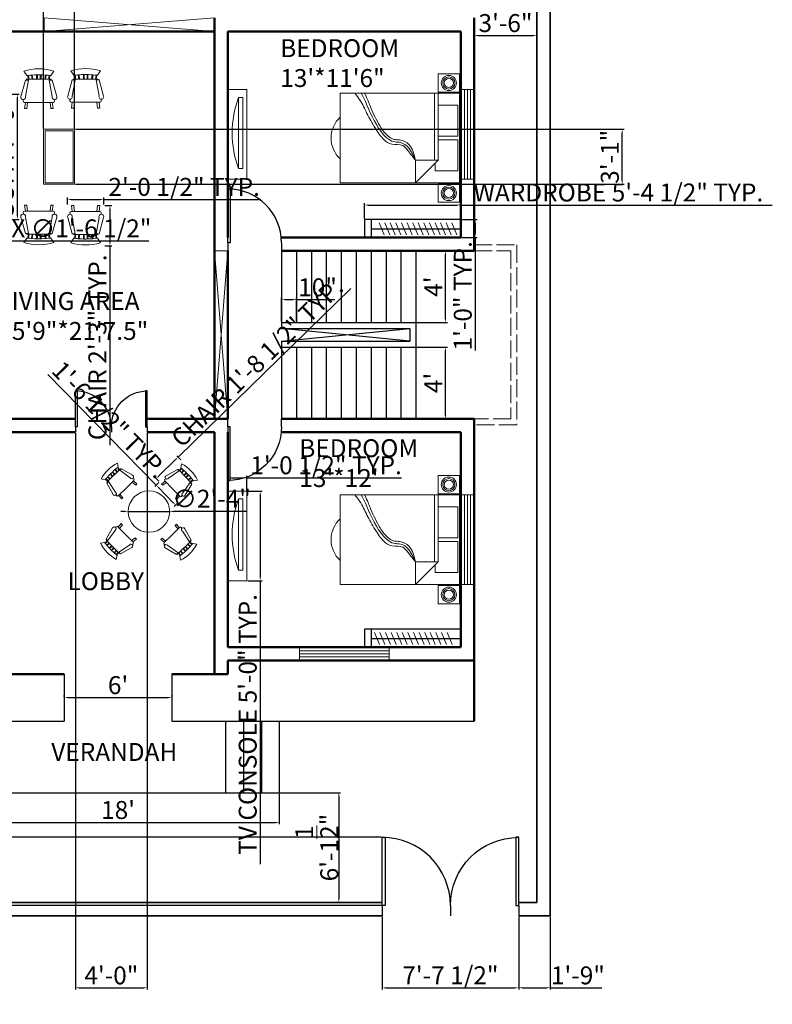
# Model space of a CAD drawing. Units: inches. Extents: x 6286 to 7213, y 5725 to 6776.
# Tile 3 of 5: x 6709 to 7213, y 5725 to 6385. Entities that reach past the tile are written whole.
import ezdxf

# ---------------------------------------------------------------- set-up
doc = ezdxf.new("R2010")
doc.units = ezdxf.units.IN
doc.linetypes.add('ACAD_ISO02W100', pattern=[15, 12, -3])
for name, color, linetype, lineweight in [('A-ANNO-DIMS', 2, 'Continuous', 18), ('A-AREA-IDEN', 7, 'Continuous', 25), ('A-DOOR', 3, 'Continuous', 25), ('A-FLOR', 7, 'Continuous', 25), ('A-FLOR-CASE', 8, 'Continuous', 25), ('A-FLOR-CASE-PATT', 252, 'Continuous', 13), ('A-FLOR-STRS', 7, 'Continuous', 25), ('A-FLOR-STRS-HIDN', 8, 'ACAD_ISO02W100', 18), ('A-FURN', 8, 'Continuous', 18), ('A-GLAZ', 4, 'Continuous', 18), ('A-WALL', 7, 'Continuous', 50), ('A-WALL-OPEN', 7, 'Continuous', 18), ('C-PROP', 7, 'Continuous', 35), ('L-SITE-GATE', 3, 'Continuous', 25)]:
    doc.layers.add(name, color=color, linetype=linetype, lineweight=lineweight)
doc.styles.get("Standard").update_dxf_attribs({"font": 'arial.ttf'})
doc.dimstyles.new('ISO-25', dxfattribs={"dimtxt": 12, "dimasz": 2.5, "dimexe": 1.25, "dimexo": 0.625, "dimtad": 1, "dimdec": 1, "dimlunit": 4, "dimtxsty": 'Standard', "dimcen": 2.5, "dimadec": 0, "dimazin": 0, "dimtfac": 1, "dimtdec": 1, "dimtmove": 0, "dimatfit": 3, "dimfxl": 1, "dimarcsym": 0})

# ---------------------------------------------------------------- blocks, each defined once
blk = doc.blocks.new('Chair - Rocking')
for p, q in [((-8, -4.5), (-10, -1.5)), ((-7.5, -4.5), (-7, -7)), ((-6.5, -7), (-7.02225, -4.43)), ((-4.5, -7), (-4.96674, -4.19951)), ((-4, -7), (-4.40532, -4.16272)), ((-1.5, -4.05012), (-1.5, -7)), ((-1, -7), (-1, -4.05012)), ((1, -7), (1, -4.04655)), ((1.5, -4.05012), (1.5, -7)), ((4, -7), (4.40187, -4.18694)), ((4.5, -7), (4.96761, -4.19437)), ((6.5, -7), (7, -4.4057)), ((7.5, -4.5), (7, -7)), ((8, -4.5), (10, -1.5)), ((-9, -7.5), (-12, -18.49999)), ((-7, -7.5), (-9, -7.5)), ((-9, -18.49999), (-7, -7.5)), ((-8.23428, -6.99939), (-8.3093, -7.47958)), ((-8.23041, -7), (8.23915, -7)), ((7, -7.5), (9, -7.5)), ((9, -18.49999), (7, -7.5)), ((8.31071, -7.48854), (8.23449, -7.00073)), ((9, -7.5), (12, -18.49999)), ((-10.36644, -20.64523), (-10.5, -21.49999)), ((-9, -22.49999), (-9.5, -26.49999)), ((0, -22.49999), (-9.5, -22.49999)), ((-8, -26.49999), (-7.5, -22.49999)), ((0, -22.49999), (9.5, -22.49999)), ((8, -26.49999), (7.5, -22.49999)), ((9, -22.49999), (9.5, -26.49999)), ((10.5, -21.49999), (10.3575, -20.58798)), ((-9.5, -26.49999), (-8, -26.49999)), ((9.5, -26.49999), (8, -26.49999))]:
    blk.add_line(p, q)
for centre, radius, start, end in [((0, -34.08333), 34.08333, 72.93847, 107.0615), ((0, -68.25004), 64.25, 93.92211, 97.15267), ((0, -68.25004), 64.25, 82.84733, 93.92211), ((-10.5, -18.99999), 1.58114, 161.5651, 18.43495), ((10.5, -18.99999), 1.58114, 161.5651, 18.43495), ((-9.5, -21.49999), 1, 180, 270), ((9.5, -21.49999), 1, 270, 0)]:
    blk.add_arc(centre, radius, start, end)
blk = doc.blocks.new('*U2')
for p, q in [((0, 0), (0, -6)), ((40, 0), (40, -6))]:
    blk.add_line(p, q)
blk.add_lwpolyline([(0, 0), (0, 40), (1.75, 40), (1.75, 0)], close=True)
blk.add_arc((0, 0), 40, 0, 90)
blk = doc.blocks.new('*D16')
at = {"layer": 'A-ANNO-DIMS', "color": 0, "lineweight": -2, "transparency": 16777216}
for p, q in [((6883.92, 6182.89), (6883.92, 6198.79)), ((6886.42, 6197.54), (6891.42, 6197.54)), ((6893.92, 6182.89), (6893.92, 6198.79)), ((6893.92, 6197.54), (6919.66, 6197.54))]:
    blk.add_line(p, q, dxfattribs=at)
at = {"layer": 'A-ANNO-DIMS', "color": 0, "lineweight": 100, "transparency": 16777216}
for points in [[(6886.42, 6197.96), (6886.42, 6197.12), (6883.92, 6197.54)], [(6891.42, 6197.96), (6891.42, 6197.12), (6893.92, 6197.54)]]:
    blk.add_solid(points, dxfattribs=at)
at = {"layer": 'Defpoints', "color": 0, "lineweight": 100, "transparency": 16777216}
for p in [(6893.92, 6197.54), (6883.92, 6182.26), (6893.92, 6182.26)]:
    blk.add_point(p, dxfattribs=at)
at = {"layer": 'A-ANNO-DIMS', "color": 0, "transparency": 16777216, "insert": (6908.04, 6204.29), "char_height": 12, "attachment_point": 5}
blk.add_mtext('10"', dxfattribs=at)
blk = doc.blocks.new('*D17')
at = {"layer": 'A-ANNO-DIMS', "color": 0, "lineweight": -2, "transparency": 16777216}
for p, q in [((6964.55, 6230.26), (6995.04, 6230.26)), ((6993.79, 6184.76), (6993.79, 6227.76)), ((6964.55, 6182.26), (6995.04, 6182.26))]:
    blk.add_line(p, q, dxfattribs=at)
at = {"layer": 'A-ANNO-DIMS', "color": 0, "lineweight": 100, "transparency": 16777216}
for points in [[(6993.38, 6227.76), (6994.21, 6227.76), (6993.79, 6230.26)], [(6993.38, 6184.76), (6994.21, 6184.76), (6993.79, 6182.26)]]:
    blk.add_solid(points, dxfattribs=at)
at = {"layer": 'Defpoints', "color": 0, "lineweight": 100, "transparency": 16777216}
for p in [(6963.92, 6230.26), (6993.79, 6230.26), (6963.92, 6182.26)]:
    blk.add_point(p, dxfattribs=at)
at = {"layer": 'A-ANNO-DIMS', "color": 0, "transparency": 16777216, "insert": (6987.17, 6206.26), "char_height": 12, "attachment_point": 5, "rotation": 90}
blk.add_mtext("4'", dxfattribs=at)
blk = doc.blocks.new('*D18')
at = {"layer": 'A-ANNO-DIMS', "color": 0, "lineweight": -2, "transparency": 16777216}
for p, q in [((6964.55, 6165.76), (6995.04, 6165.76)), ((6993.79, 6120.26), (6993.79, 6163.26)), ((6964.55, 6117.76), (6995.04, 6117.76))]:
    blk.add_line(p, q, dxfattribs=at)
at = {"layer": 'A-ANNO-DIMS', "color": 0, "lineweight": 100, "transparency": 16777216}
for points in [[(6993.38, 6163.26), (6994.21, 6163.26), (6993.79, 6165.76)], [(6993.38, 6120.26), (6994.21, 6120.26), (6993.79, 6117.76)]]:
    blk.add_solid(points, dxfattribs=at)
at = {"layer": 'Defpoints', "color": 0, "lineweight": 100, "transparency": 16777216}
for p in [(6963.92, 6165.76), (6993.79, 6165.76), (6963.92, 6117.76)]:
    blk.add_point(p, dxfattribs=at)
at = {"layer": 'A-ANNO-DIMS', "color": 0, "transparency": 16777216, "insert": (6987.17, 6141.76), "char_height": 12, "attachment_point": 5, "rotation": 90}
blk.add_mtext("4'", dxfattribs=at)
blk = doc.blocks.new('*D20')
at = {"layer": 'A-ANNO-DIMS', "color": 0, "lineweight": -2, "transparency": 16777216}
for p, q in [((6666.42, 5866.64), (6666.42, 5846.12)), ((6882.42, 5866.64), (6882.42, 5846.12)), ((6668.92, 5847.37), (6879.92, 5847.37))]:
    blk.add_line(p, q, dxfattribs=at)
at = {"layer": 'A-ANNO-DIMS', "color": 0, "lineweight": 100, "transparency": 16777216}
for points in [[(6668.92, 5847.78), (6668.92, 5846.95), (6666.42, 5847.37)], [(6879.92, 5847.78), (6879.92, 5846.95), (6882.42, 5847.37)]]:
    blk.add_solid(points, dxfattribs=at)
at = {"layer": 'Defpoints', "color": 0, "lineweight": 100, "transparency": 16777216}
for p in [(6666.42, 5867.26), (6882.42, 5867.26), (6882.42, 5847.37)]:
    blk.add_point(p, dxfattribs=at)
at = {"layer": 'A-ANNO-DIMS', "color": 0, "transparency": 16777216, "insert": (6774.42, 5854.12), "char_height": 12, "attachment_point": 5}
blk.add_mtext("18'", dxfattribs=at)
blk = doc.blocks.new('*D21')
at = {"layer": 'A-ANNO-DIMS', "color": 0, "lineweight": -2, "transparency": 16777216}
for p, q in [((6738.42, 5931.64), (6738.42, 5932.26)), ((6740.92, 5931.01), (6807.92, 5931.01)), ((6810.42, 5931.64), (6810.42, 5932.26))]:
    blk.add_line(p, q, dxfattribs=at)
at = {"layer": 'A-ANNO-DIMS', "color": 0, "lineweight": 100, "transparency": 16777216}
for points in [[(6740.92, 5931.43), (6740.92, 5930.6), (6738.42, 5931.01)], [(6807.92, 5931.43), (6807.92, 5930.6), (6810.42, 5931.01)]]:
    blk.add_solid(points, dxfattribs=at)
at = {"layer": 'Defpoints', "color": 0, "lineweight": 100, "transparency": 16777216}
for p in [(6738.42, 5931.01), (6810.42, 5931.01), (6810.42, 5931.01)]:
    blk.add_point(p, dxfattribs=at)
at = {"layer": 'A-ANNO-DIMS', "color": 0, "transparency": 16777216, "insert": (6774.42, 5937.77), "char_height": 12, "attachment_point": 5}
blk.add_mtext("6'", dxfattribs=at)
blk = doc.blocks.new('*D22')
at = {"layer": 'A-ANNO-DIMS', "color": 0, "lineweight": -2, "transparency": 16777216}
for p, q in [((6883.05, 5867.26), (6923.5, 5867.26)), ((6922.25, 5864.76), (6922.25, 5796.26)), ((6883.05, 5793.76), (6923.5, 5793.76))]:
    blk.add_line(p, q, dxfattribs=at)
at = {"layer": 'A-ANNO-DIMS', "color": 0, "lineweight": 100, "transparency": 16777216}
for points in [[(6921.84, 5864.76), (6922.67, 5864.76), (6922.25, 5867.26)], [(6921.84, 5796.26), (6922.67, 5796.26), (6922.25, 5793.76)]]:
    blk.add_solid(points, dxfattribs=at)
at = {"layer": 'Defpoints', "color": 0, "lineweight": 100, "transparency": 16777216}
for p in [(6882.42, 5867.26), (6882.42, 5793.76), (6922.25, 5793.76)]:
    blk.add_point(p, dxfattribs=at)
at = {"layer": 'A-ANNO-DIMS', "color": 0, "transparency": 16777216, "insert": (6907.48, 5830.51), "char_height": 12, "attachment_point": 5, "rotation": 90}
blk.add_mtext('6\'-1{\\H1x;\\S1/2;}"', dxfattribs=at)
blk = doc.blocks.new('*D24')
at = {"layer": 'A-ANNO-DIMS', "color": 0, "lineweight": -2, "transparency": 16777216}
for p, q in [((7012.92, 6385.64), (7012.92, 6373.28)), ((7054.92, 6385.64), (7054.92, 6373.28)), ((7015.42, 6374.53), (7052.42, 6374.53))]:
    blk.add_line(p, q, dxfattribs=at)
at = {"layer": 'A-ANNO-DIMS', "color": 0, "lineweight": 100, "transparency": 16777216}
for points in [[(7015.42, 6374.95), (7015.42, 6374.12), (7012.92, 6374.53)], [(7052.42, 6374.95), (7052.42, 6374.12), (7054.92, 6374.53)]]:
    blk.add_solid(points, dxfattribs=at)
at = {"layer": 'Defpoints', "color": 0, "lineweight": 100, "transparency": 16777216}
for p in [(7012.92, 6386.26), (7054.92, 6386.26), (7054.92, 6374.53)]:
    blk.add_point(p, dxfattribs=at)
at = {"layer": 'A-ANNO-DIMS', "color": 0, "transparency": 16777216, "insert": (7033.92, 6381.29), "char_height": 12, "attachment_point": 5}
blk.add_mtext('3\'-6"', dxfattribs=at)
blk = doc.blocks.new('WIN-60IN')
for p, q in [((0, 9), (0, 0)), ((60, 0), (60, 9)), ((60, 6.5), (0, 6.5)), ((60, 4.5), (0, 4.5)), ((60, 2.5), (0, 2.5))]:
    blk.add_line(p, q)
blk = doc.blocks.new('NIGHTSTAND-LAMP')
blk.add_lwpolyline([(12.23, 14.4), (0, 14.4), (0, 0), (12.23, 0)], close=True)
for radius in [5.06, 4.06, 3.06]:
    blk.add_circle((6.12, 7.2), radius)
blk = doc.blocks.new('TV-CONSOLE-60IN')
for points in [[(0, 12.71), (60, 12.71), (60, 0), (0, 0)], [(5.19, 10.13), (52.94, 10.13), (52.94, 7.18), (5.19, 7.18)]]:
    blk.add_lwpolyline(points, close=True)
blk.add_arc((29.07, 71.71), 68.81, 249.69468, 290.30532)
blk = doc.blocks.new('Bed - Queen')
for p, q in [((0, -80.00003), (0, 0)), ((0, 0), (59.99999, 0)), ((59.99999, 0), (59.99999, -80.00003)), ((7.99999, -1.2), (28.79998, -1.2)), ((7.99999, -14.4), (7.99999, -1.2)), ((28.79998, -1.2), (28.79998, -14.4)), ((31.19999, -1.2), (51.99999, -1.2)), ((31.19999, -14.4), (31.19999, -1.2)), ((51.99999, -1.2), (51.99999, -16.4)), ((0, -14.4), (44.8, -14.4)), ((44.8, -16.8), (0, -16.8)), ((59.99999, -29.6), (44.8, -14.4)), ((44.8, -14.4), (44.8, -29.6)), ((51.99999, -16.4), (46.79936, -16.4)), ((44.8, -29.6), (59.99999, -29.6)), ((59.99999, -80.00003), (0, -80.00003))]:
    blk.add_line(p, q)
blk = doc.blocks.new('BED-QUEEN-DRESSED')
blk.add_arc((30, 18.96), 18.96, 222.75176, 317.24824)
for points, knots in [([(44.8, 56.49), (39.19, 53.96), (32.77, 51.07), (32.71, 32.08), (7.2, 24.53), (0, 20.27)], [0, 0, 0, 0, 16.08431, 18.417841, 48.068097, 48.068097, 48.068097, 48.068097]), ([(44.8, 56.49), (41.02, 55.65), (34.77, 54.26), (30.9, 47.2), (31.38, 41.03), (26.76, 35.63), (19.36, 31.03), (9.68, 26.38), (4.48, 24.69), (0, 22.46)], [0, 0, 0, 0, 11.066231, 18.341473, 21.645482, 29.256421, 37.126455, 49.94498, 57.001864, 57.001864, 57.001864, 57.001864]), ([(44.8, 56.49), (42.82, 54.88), (39.55, 52.2), (33.5, 47.94), (35.23, 40.79), (30.55, 34.13), (23.14, 29.37), (13.11, 23.54), (6.2, 20.75), (1.43, 17.09), (0, 16.03)], [0, 0, 0, 0, 7.83924, 12.978287, 20.287315, 26.568624, 36.127852, 46.548326, 57.45004, 62.118815, 62.118815, 62.118815, 62.118815])]:
    blk.add_open_spline(points, degree=3, knots=knots)
blk.add_blockref('Bed - Queen', (0, 86.09))
blk = doc.blocks.new('WARDROBE-RETURN-RAIL')
for p, q in [((0, 64.5), (0, 0)), ((6.49, 64.5), (6.49, 4.5)), ((0, 4.5), (12, 4.5)), ((0, 0), (12, 0))]:
    blk.add_line(p, q)
blk = doc.blocks.new('*D39')
at = {"layer": 'A-ANNO-DIMS', "color": 0, "lineweight": -2, "transparency": 16777216}
for p, q in [((6765.53, 6260.66), (6770.21, 6260.66)), ((6768.96, 6258.16), (6768.96, 6236.16)), ((6765.53, 6233.66), (6770.21, 6233.66)), ((6768.96, 6233.66), (6768.96, 6100.08))]:
    blk.add_line(p, q, dxfattribs=at)
at = {"layer": 'A-ANNO-DIMS', "color": 0, "lineweight": 100, "transparency": 16777216}
for points in [[(6768.54, 6258.16), (6769.37, 6258.16), (6768.96, 6260.66)], [(6768.54, 6236.16), (6769.37, 6236.16), (6768.96, 6233.66)]]:
    blk.add_solid(points, dxfattribs=at)
at = {"layer": 'Defpoints', "color": 0, "lineweight": 100, "transparency": 16777216}
for p in [(6764.91, 6260.66), (6764.91, 6233.66), (6768.96, 6233.66)]:
    blk.add_point(p, dxfattribs=at)
at = {"layer": 'A-ANNO-DIMS', "color": 0, "transparency": 16777216, "insert": (6762.12, 6165.62), "char_height": 12, "attachment_point": 5, "rotation": 90}
blk.add_mtext('CHAIR 2\'-3" TYP.', dxfattribs=at)
blk = doc.blocks.new('*D40')
at = {"layer": 'A-ANNO-DIMS', "color": 0, "lineweight": -2, "transparency": 16777216}
for p, q in [((6740.47, 6261.28), (6740.47, 6265.96)), ((6742.97, 6264.71), (6762.41, 6264.71)), ((6764.91, 6261.28), (6764.91, 6265.96)), ((6764.91, 6264.71), (6869.97, 6264.71))]:
    blk.add_line(p, q, dxfattribs=at)
at = {"layer": 'A-ANNO-DIMS', "color": 0, "lineweight": 100, "transparency": 16777216}
for points in [[(6742.97, 6265.12), (6742.97, 6264.29), (6740.47, 6264.71)], [(6762.41, 6265.12), (6762.41, 6264.29), (6764.91, 6264.71)]]:
    blk.add_solid(points, dxfattribs=at)
at = {"layer": 'Defpoints', "color": 0, "lineweight": 100, "transparency": 16777216}
for p in [(6740.47, 6260.66), (6764.91, 6264.71), (6764.91, 6260.66)]:
    blk.add_point(p, dxfattribs=at)
at = {"layer": 'A-ANNO-DIMS', "color": 0, "transparency": 16777216, "insert": (6818.69, 6271.54), "char_height": 12, "attachment_point": 5}
blk.add_mtext('2\'-0 1/2" TYP.', dxfattribs=at)
blk = doc.blocks.new('*D41')
at = {"layer": 'A-ANNO-DIMS', "color": 0, "lineweight": -2, "transparency": 16777216}
for p, q in [((6814.71, 6092.11), (6930.26, 6205)), ((6801.73, 6079.43), (6812.92, 6090.37)), ((6816.44, 6090.34), (6813.84, 6093.01)), ((6801.67, 6075.92), (6799.07, 6078.58))]:
    blk.add_line(p, q, dxfattribs=at)
at = {"layer": 'A-ANNO-DIMS', "color": 0, "lineweight": 100, "transparency": 16777216}
for points in [[(6812.63, 6090.66), (6813.21, 6090.07), (6814.71, 6092.11)], [(6801.44, 6079.73), (6802.02, 6079.13), (6799.94, 6077.68)]]:
    blk.add_solid(points, dxfattribs=at)
at = {"layer": 'Defpoints', "color": 0, "lineweight": 100, "transparency": 16777216}
for p in [(6814.71, 6092.11), (6816.88, 6089.9), (6802.11, 6075.47)]:
    blk.add_point(p, dxfattribs=at)
at = {"layer": 'A-ANNO-DIMS', "color": 0, "transparency": 16777216, "insert": (6868.61, 6154.31), "char_height": 12, "attachment_point": 5, "rotation": 44.33278}
blk.add_mtext('CHAIR 1\'-8 1/2" TYP.', dxfattribs=at)
blk = doc.blocks.new('*D42')
at = {"layer": 'A-ANNO-DIMS', "color": 0, "lineweight": -2, "transparency": 16777216}
for p, q in [((6799.89, 6073.3), (6727.4, 6147.5)), ((6801.66, 6075.03), (6799, 6072.43)), ((6811.2, 6061.73), (6801.64, 6071.52)), ((6814.72, 6061.67), (6812.06, 6059.07))]:
    blk.add_line(p, q, dxfattribs=at)
at = {"layer": 'A-ANNO-DIMS', "color": 0, "lineweight": 100, "transparency": 16777216}
for points in [[(6801.94, 6071.81), (6801.34, 6071.23), (6799.89, 6073.3)], [(6811.5, 6062.02), (6810.9, 6061.44), (6812.95, 6059.94)]]:
    blk.add_solid(points, dxfattribs=at)
at = {"layer": 'Defpoints', "color": 0, "lineweight": 100, "transparency": 16777216}
for p in [(6802.11, 6075.47), (6799.89, 6073.3), (6815.17, 6062.1)]:
    blk.add_point(p, dxfattribs=at)
at = {"layer": 'A-ANNO-DIMS', "color": 0, "transparency": 16777216, "insert": (6767.66, 6116.07), "char_height": 12, "attachment_point": 5, "rotation": 314.33278}
blk.add_mtext('1\'-6 1/2" TYP.', dxfattribs=at)
blk = doc.blocks.new('*D45')
at = {"layer": 'A-ANNO-DIMS', "color": 0, "lineweight": -2, "transparency": 16777216}
for p, q in [((6861.26, 6069.22), (6870.89, 6069.22)), ((6869.64, 6066.72), (6869.64, 6011.72)), ((6861.26, 6009.22), (6870.89, 6009.22)), ((6869.64, 6009.22), (6869.64, 5819.3))]:
    blk.add_line(p, q, dxfattribs=at)
at = {"layer": 'A-ANNO-DIMS', "color": 0, "lineweight": 100, "transparency": 16777216}
for points in [[(6869.22, 6066.72), (6870.05, 6066.72), (6869.64, 6069.22)], [(6869.22, 6011.72), (6870.05, 6011.72), (6869.64, 6009.22)]]:
    blk.add_solid(points, dxfattribs=at)
at = {"layer": 'Defpoints', "color": 0, "lineweight": 100, "transparency": 16777216}
for p in [(6860.64, 6069.22), (6860.64, 6009.22), (6869.64, 6009.22)]:
    blk.add_point(p, dxfattribs=at)
at = {"layer": 'A-ANNO-DIMS', "color": 0, "transparency": 16777216, "insert": (6862.8, 5913.01), "char_height": 12, "attachment_point": 5, "rotation": 90}
blk.add_mtext('TV CONSOLE 5\'-0" TYP.', dxfattribs=at)
blk = doc.blocks.new('*D46')
at = {"layer": 'A-ANNO-DIMS', "color": 0, "lineweight": -2, "transparency": 16777216}
for p, q in [((6847.92, 6069.84), (6847.92, 6079.47)), ((6850.42, 6078.22), (6858.14, 6078.22)), ((6860.64, 6069.84), (6860.64, 6079.47)), ((6860.64, 6078.22), (6964.36, 6078.22))]:
    blk.add_line(p, q, dxfattribs=at)
at = {"layer": 'A-ANNO-DIMS', "color": 0, "lineweight": 100, "transparency": 16777216}
for points in [[(6850.42, 6078.63), (6850.42, 6077.8), (6847.92, 6078.22)], [(6858.14, 6078.63), (6858.14, 6077.8), (6860.64, 6078.22)]]:
    blk.add_solid(points, dxfattribs=at)
at = {"layer": 'Defpoints', "color": 0, "lineweight": 100, "transparency": 16777216}
for p in [(6860.64, 6078.22), (6847.92, 6069.22), (6860.64, 6069.22)]:
    blk.add_point(p, dxfattribs=at)
at = {"layer": 'A-ANNO-DIMS', "color": 0, "transparency": 16777216, "insert": (6913.75, 6085.05), "char_height": 12, "attachment_point": 5}
blk.add_mtext('1\'-0 1/2" TYP.', dxfattribs=at)
blk = doc.blocks.new('*D49')
at = {"layer": 'A-ANNO-DIMS', "color": 0, "lineweight": -2, "transparency": 16777216}
for p, q in [((6939.42, 6251.89), (6939.42, 6262.19)), ((6941.92, 6260.94), (7001.42, 6260.94)), ((7003.92, 6251.89), (7003.92, 6262.19)), ((7003.92, 6260.94), (7212.66, 6260.94))]:
    blk.add_line(p, q, dxfattribs=at)
at = {"layer": 'A-ANNO-DIMS', "color": 0, "lineweight": 100, "transparency": 16777216}
for points in [[(6941.92, 6261.36), (6941.92, 6260.53), (6939.42, 6260.94)], [(7001.42, 6261.36), (7001.42, 6260.53), (7003.92, 6260.94)]]:
    blk.add_solid(points, dxfattribs=at)
at = {"layer": 'Defpoints', "color": 0, "lineweight": 100, "transparency": 16777216}
for p in [(7003.92, 6260.94), (6939.42, 6251.27), (7003.92, 6251.27)]:
    blk.add_point(p, dxfattribs=at)
at = {"layer": 'A-ANNO-DIMS', "color": 0, "transparency": 16777216, "insert": (7109.54, 6267.78), "char_height": 12, "attachment_point": 5}
blk.add_mtext('WARDROBE 5\'-4 1/2" TYP.', dxfattribs=at)
blk = doc.blocks.new('*D50')
at = {"layer": 'A-ANNO-DIMS', "color": 0, "lineweight": -2, "transparency": 16777216}
for p, q in [((7004.55, 6251.27), (7014.85, 6251.27)), ((7013.6, 6248.77), (7013.6, 6241.76)), ((7004.55, 6239.26), (7014.85, 6239.26)), ((7013.6, 6239.26), (7013.6, 6163.5))]:
    blk.add_line(p, q, dxfattribs=at)
at = {"layer": 'A-ANNO-DIMS', "color": 0, "lineweight": 100, "transparency": 16777216}
for points in [[(7013.18, 6248.77), (7014.02, 6248.77), (7013.6, 6251.27)], [(7013.18, 6241.76), (7014.02, 6241.76), (7013.6, 6239.26)]]:
    blk.add_solid(points, dxfattribs=at)
at = {"layer": 'Defpoints', "color": 0, "lineweight": 100, "transparency": 16777216}
for p in [(7003.92, 6251.27), (7003.92, 6239.26), (7013.6, 6239.26)]:
    blk.add_point(p, dxfattribs=at)
at = {"layer": 'A-ANNO-DIMS', "color": 0, "transparency": 16777216, "insert": (7006.85, 6200.13), "char_height": 12, "attachment_point": 5, "rotation": 90}
blk.add_mtext('1\'-0" TYP.', dxfattribs=at)
blk = doc.blocks.new('*D53')
at = {"layer": 'A-ANNO-DIMS', "color": 0, "lineweight": -2, "transparency": 16777216}
for p, q in [((6694.98, 6335.25), (6708.2, 6335.25)), ((6706.95, 6253.75), (6706.95, 6332.75)), ((6694.98, 6251.25), (6708.2, 6251.25))]:
    blk.add_line(p, q, dxfattribs=at)
at = {"layer": 'A-ANNO-DIMS', "color": 0, "lineweight": 100, "transparency": 16777216}
for points in [[(6706.54, 6332.75), (6707.37, 6332.75), (6706.95, 6335.25)], [(6706.54, 6253.75), (6707.37, 6253.75), (6706.95, 6251.25)]]:
    blk.add_solid(points, dxfattribs=at)
at = {"layer": 'Defpoints', "color": 0, "lineweight": 100, "transparency": 16777216}
for p in [(6694.35, 6335.25), (6706.95, 6335.25), (6694.35, 6251.25)]:
    blk.add_point(p, dxfattribs=at)
at = {"layer": 'A-ANNO-DIMS', "color": 0, "transparency": 16777216, "insert": (6700.12, 6293.25), "char_height": 12, "attachment_point": 5, "rotation": 90}
blk.add_mtext('SOFA 7\'-0"', dxfattribs=at)
blk = doc.blocks.new('*D62')
at = {"layer": 'A-ANNO-DIMS', "color": 0, "lineweight": -2, "transparency": 16777216}
for p, q in [((6951.28, 5784.14), (6951.28, 5735.31)), ((7042.76, 5784.14), (7042.76, 5735.31)), ((6953.78, 5736.56), (7040.26, 5736.56))]:
    blk.add_line(p, q, dxfattribs=at)
at = {"layer": 'A-ANNO-DIMS', "color": 0, "lineweight": 100, "transparency": 16777216}
for points in [[(6953.78, 5736.98), (6953.78, 5736.15), (6951.28, 5736.56)], [(7040.26, 5736.98), (7040.26, 5736.15), (7042.76, 5736.56)]]:
    blk.add_solid(points, dxfattribs=at)
at = {"layer": 'Defpoints', "color": 0, "lineweight": 100, "transparency": 16777216}
for p in [(6951.28, 5784.76), (7042.76, 5784.76), (7042.76, 5736.56)]:
    blk.add_point(p, dxfattribs=at)
at = {"layer": 'A-ANNO-DIMS', "color": 0, "transparency": 16777216, "insert": (6997.02, 5743.39), "char_height": 12, "attachment_point": 5}
blk.add_mtext('7\'-7 1/2"', dxfattribs=at)
blk = doc.blocks.new('*D63')
at = {"layer": 'A-ANNO-DIMS', "color": 0, "lineweight": -2, "transparency": 16777216}
for p, q in [((7042.76, 5784.14), (7042.76, 5735.31)), ((7063.92, 5784.14), (7063.92, 5735.31)), ((7045.26, 5736.56), (7061.42, 5736.56)), ((7063.92, 5736.56), (7098.44, 5736.56))]:
    blk.add_line(p, q, dxfattribs=at)
at = {"layer": 'A-ANNO-DIMS', "color": 0, "lineweight": 100, "transparency": 16777216}
for points in [[(7045.26, 5736.98), (7045.26, 5736.15), (7042.76, 5736.56)], [(7061.42, 5736.98), (7061.42, 5736.15), (7063.92, 5736.56)]]:
    blk.add_solid(points, dxfattribs=at)
at = {"layer": 'Defpoints', "color": 0, "lineweight": 100, "transparency": 16777216}
for p in [(7042.76, 5784.76), (7063.92, 5784.76), (7063.92, 5736.56)]:
    blk.add_point(p, dxfattribs=at)
at = {"layer": 'A-ANNO-DIMS', "color": 0, "transparency": 16777216, "insert": (7082.43, 5743.32), "char_height": 12, "attachment_point": 5}
blk.add_mtext('1\'-9"', dxfattribs=at)
blk = doc.blocks.new('*D64')
at = {"layer": 'A-ANNO-DIMS', "color": 0, "lineweight": -2, "transparency": 16777216}
for p, q in [((6724.5, 6312.3), (6724.5, 6762.71)), ((6727, 6761.46), (6742.8, 6761.46)), ((6745.3, 6312.3), (6745.3, 6762.71)), ((6745.3, 6761.46), (6779.82, 6761.46))]:
    blk.add_line(p, q, dxfattribs=at)
at = {"layer": 'A-ANNO-DIMS', "color": 0, "lineweight": 100, "transparency": 16777216}
for points in [[(6727, 6761.88), (6727, 6761.05), (6724.5, 6761.46)], [(6742.8, 6761.88), (6742.8, 6761.05), (6745.3, 6761.46)]]:
    blk.add_solid(points, dxfattribs=at)
at = {"layer": 'Defpoints', "color": 0, "lineweight": 100, "transparency": 16777216}
for p in [(6745.3, 6761.46), (6724.5, 6311.67), (6745.3, 6311.67)]:
    blk.add_point(p, dxfattribs=at)
at = {"layer": 'A-ANNO-DIMS', "color": 0, "transparency": 16777216, "insert": (6763.81, 6768.22), "char_height": 12, "attachment_point": 5}
blk.add_mtext('1\'-9"', dxfattribs=at)
blk = doc.blocks.new('*D65')
at = {"layer": 'A-ANNO-DIMS', "color": 0, "lineweight": -2, "transparency": 16777216}
for p, q in [((6745.93, 6311.67), (7113.37, 6311.67)), ((7112.12, 6277.32), (7112.12, 6309.17)), ((6745.93, 6274.82), (7113.37, 6274.82))]:
    blk.add_line(p, q, dxfattribs=at)
at = {"layer": 'A-ANNO-DIMS', "color": 0, "lineweight": 100, "transparency": 16777216}
for points in [[(7111.71, 6309.17), (7112.54, 6309.17), (7112.12, 6311.67)], [(7111.71, 6277.32), (7112.54, 6277.32), (7112.12, 6274.82)]]:
    blk.add_solid(points, dxfattribs=at)
at = {"layer": 'Defpoints', "color": 0, "lineweight": 100, "transparency": 16777216}
for p in [(6745.3, 6311.67), (7112.12, 6311.67), (6745.3, 6274.82)]:
    blk.add_point(p, dxfattribs=at)
at = {"layer": 'A-ANNO-DIMS', "color": 0, "transparency": 16777216, "insert": (7105.37, 6293.25), "char_height": 12, "attachment_point": 5, "rotation": 90}
blk.add_mtext('3\'-1"', dxfattribs=at)
blk = doc.blocks.new('*D66')
at = {"layer": 'A-ANNO-DIMS', "color": 0, "lineweight": -2, "transparency": 16777216}
for p, q in [((6745.92, 6108.14), (6745.92, 5735.31)), ((6793.92, 6108.14), (6793.92, 5735.31)), ((6748.42, 5736.56), (6791.42, 5736.56))]:
    blk.add_line(p, q, dxfattribs=at)
at = {"layer": 'A-ANNO-DIMS', "color": 0, "lineweight": 100, "transparency": 16777216}
for points in [[(6748.42, 5736.98), (6748.42, 5736.15), (6745.92, 5736.56)], [(6791.42, 5736.98), (6791.42, 5736.15), (6793.92, 5736.56)]]:
    blk.add_solid(points, dxfattribs=at)
at = {"layer": 'Defpoints', "color": 0, "lineweight": 100, "transparency": 16777216}
for p in [(6745.92, 6108.76), (6793.92, 6108.76), (6793.92, 5736.56)]:
    blk.add_point(p, dxfattribs=at)
at = {"layer": 'A-ANNO-DIMS', "color": 0, "transparency": 16777216, "insert": (6769.92, 5743.32), "char_height": 12, "attachment_point": 5}
blk.add_mtext('4\'-0"', dxfattribs=at)
blk = doc.blocks.new('*D74')
at = {"layer": 'A-ANNO-DIMS', "color": 0, "lineweight": -2, "transparency": 16777216}
for p, q in [((6310.72, 5837.37), (6310.72, 5900.97)), ((6950.65, 5837.37), (6309.47, 5837.37)), ((6310.72, 5794.12), (6310.72, 5834.87)), ((6950.65, 5791.62), (6309.47, 5791.62))]:
    blk.add_line(p, q, dxfattribs=at)
at = {"layer": 'A-ANNO-DIMS', "color": 0, "lineweight": 100, "transparency": 16777216}
for points in [[(6310.31, 5834.87), (6311.14, 5834.87), (6310.72, 5837.37)], [(6310.31, 5794.12), (6311.14, 5794.12), (6310.72, 5791.62)]]:
    blk.add_solid(points, dxfattribs=at)
at = {"layer": 'Defpoints', "color": 0, "lineweight": 100, "transparency": 16777216}
for p in [(6310.72, 5837.37), (6951.28, 5837.37), (6951.28, 5791.62)]:
    blk.add_point(p, dxfattribs=at)
at = {"layer": 'A-ANNO-DIMS', "color": 0, "transparency": 16777216, "insert": (6303.89, 5870.42), "char_height": 12, "attachment_point": 5, "rotation": 90}
blk.add_mtext('3\'-9 1/2"', dxfattribs=at)
blk = doc.blocks.new('*D75')
at = {"layer": 'A-ANNO-DIMS', "color": 0, "lineweight": -2, "transparency": 16777216}
for p, q in [((6669.69, 6236.66), (6667.19, 6236.66)), ((6672.19, 6236.66), (6690.52, 6236.66)), ((6795.04, 6236.67), (6693.02, 6236.66))]:
    blk.add_line(p, q, dxfattribs=at)
at = {"layer": 'A-ANNO-DIMS', "color": 0, "lineweight": 100, "transparency": 16777216}
for points in [[(6669.69, 6237.08), (6669.69, 6236.25), (6672.19, 6236.66)], [(6693.02, 6237.08), (6693.02, 6236.25), (6690.52, 6236.66)]]:
    blk.add_solid(points, dxfattribs=at)
at = {"layer": 'Defpoints', "color": 0, "lineweight": 100, "transparency": 16777216}
for p in [(6672.19, 6236.66), (6690.52, 6236.66)]:
    blk.add_point(p, dxfattribs=at)
at = {"layer": 'A-ANNO-DIMS', "color": 0, "transparency": 16777216, "insert": (6745.28, 6243.75), "char_height": 12, "attachment_point": 5, "rotation": 0.00133}
blk.add_mtext('2X ∅1\'-6 1/2"', dxfattribs=at)
blk = doc.blocks.new('*D76')
at = {"layer": 'A-ANNO-DIMS', "color": 0, "lineweight": -2, "transparency": 16777216}
for p, q in [((6778.72, 6055.57), (6776.22, 6055.57)), ((6781.22, 6055.57), (6808.99, 6055.57)), ((6860.19, 6055.57), (6811.49, 6055.57))]:
    blk.add_line(p, q, dxfattribs=at)
at = {"layer": 'A-ANNO-DIMS', "color": 0, "lineweight": 100, "transparency": 16777216}
for points in [[(6778.72, 6055.98), (6778.72, 6055.15), (6781.22, 6055.57)], [(6811.49, 6055.98), (6811.49, 6055.15), (6808.99, 6055.57)]]:
    blk.add_solid(points, dxfattribs=at)
at = {"layer": 'Defpoints', "color": 0, "lineweight": 100, "transparency": 16777216}
for p in [(6781.22, 6055.57), (6808.99, 6055.57)]:
    blk.add_point(p, dxfattribs=at)
at = {"layer": 'A-ANNO-DIMS', "color": 0, "transparency": 16777216, "insert": (6837.09, 6062.65), "char_height": 12, "attachment_point": 5, "rotation": 359.99806}
blk.add_mtext('∅2\'-4"', dxfattribs=at)

msp = doc.modelspace()

# ---------------------------------------------------------------- hatches: boundary and pattern name
at = {"layer": 'A-FLOR-CASE-PATT'}
h = msp.add_hatch(dxfattribs=at)
h.set_pattern_fill('ANSI31', color=256, scale=1.091306, angle=67.364, style=0)
h.paths.add_polyline_path([(6945.83, 6249.07), (6949.18, 6240.93), (7001.63, 6240.93), (6998.28, 6249.07)])
h = msp.add_hatch(dxfattribs=at)
h.set_pattern_fill('ANSI31', color=256, scale=1.091306, angle=67.364, style=0)
h.paths.add_polyline_path([(6945.83, 5974.57), (6949.18, 5966.43), (7001.63, 5966.43), (6998.28, 5974.57)])

# ---------------------------------------------------------------- linework, layer by layer
at = {"layer": 'A-FLOR'}
for p, q in [((6738.42, 5946.76), (6738.42, 5915.26)), ((6810.42, 5946.76), (6810.42, 5915.26)), ((6514.92, 5915.26), (6738.42, 5915.26)), ((6810.42, 5915.26), (7012.92, 5915.26))]:
    msp.add_line(p, q, dxfattribs=at)
at = {"layer": 'A-FLOR-STRS'}
for p, q in [((6883.92, 6230.26), (6883.92, 6178.26)), ((6893.92, 6230.26), (6893.92, 6182.26)), ((6903.92, 6230.26), (6903.92, 6182.26)), ((6913.92, 6230.26), (6913.92, 6182.26)), ((6923.92, 6230.26), (6923.92, 6182.26)), ((6933.92, 6230.26), (6933.92, 6182.26)), ((6943.92, 6230.26), (6943.92, 6182.26)), ((6953.92, 6230.26), (6953.92, 6182.26)), ((6963.92, 6230.26), (6963.92, 6182.26)), ((6973.92, 6230.26), (6973.92, 6117.76)), ((6883.92, 6182.26), (6973.92, 6182.26)), ((6883.92, 6178.26), (6969.92, 6178.26)), ((6883.92, 6169.76), (6969.92, 6178.26)), ((6969.92, 6169.76), (6883.92, 6178.26)), ((6969.92, 6178.26), (6969.92, 6169.76)), ((6883.92, 6169.76), (6883.92, 6117.76)), ((6883.92, 6169.76), (6969.92, 6169.76)), ((6883.92, 6165.76), (6973.92, 6165.76)), ((6893.92, 6165.76), (6893.92, 6117.76)), ((6903.92, 6165.76), (6903.92, 6117.76)), ((6913.92, 6165.76), (6913.92, 6117.76)), ((6923.92, 6165.76), (6923.92, 6117.76)), ((6933.92, 6165.76), (6933.92, 6117.76)), ((6943.92, 6165.76), (6943.92, 6117.76)), ((6953.92, 6165.76), (6953.92, 6117.76)), ((6963.92, 6165.76), (6963.92, 6117.76)), ((6846.42, 5915.26), (6846.42, 5867.26)), ((6858.42, 5915.26), (6858.42, 5867.26)), ((6870.42, 5915.26), (6870.42, 5867.26)), ((6882.42, 5915.26), (6882.42, 5867.26)), ((6666.42, 5867.26), (6882.42, 5867.26))]:
    msp.add_line(p, q, dxfattribs=at)
at = {"layer": 'A-FLOR-STRS-HIDN'}
for p, q in [((7012.92, 6234.26), (7041.58, 6234.26)), ((7041.58, 6234.26), (7041.58, 6113.76)), ((7012.92, 6230.26), (7037.58, 6230.26)), ((7037.58, 6230.26), (7037.58, 6117.76)), ((7037.58, 6117.76), (7012.92, 6117.76)), ((7041.58, 6113.76), (7012.92, 6113.76))]:
    msp.add_line(p, q, dxfattribs=at)
at = {"layer": 'A-FURN'}
for points in [[(6724.5, 6311.67), (6745.3, 6311.67), (6745.3, 6274.82), (6724.5, 6274.82)], [(6725.5, 6310.67), (6744.3, 6310.67), (6744.3, 6275.82), (6725.5, 6275.82)]]:
    msp.add_lwpolyline(points, close=True, dxfattribs=at)
msp.add_circle((6795.11, 6055.57), 13.88, dxfattribs=at)
at = {"layer": 'A-WALL'}
for p, q in [((6838.92, 6386.26), (6838.92, 6117.76)), ((7012.92, 6386.26), (7012.92, 6230.26)), ((6649.92, 6377.26), (6838.92, 6377.26)), ((6847.92, 6377.26), (6847.92, 6239.26)), ((6847.92, 6377.26), (7003.92, 6377.26)), ((7003.92, 6377.26), (7003.92, 6239.26)), ((6883.74, 6239.26), (7003.92, 6239.26)), ((6847.92, 6230.26), (6847.92, 6117.76)), ((6883.92, 6230.26), (7012.92, 6230.26)), ((6640.92, 6117.76), (6745.92, 6117.76)), ((6793.92, 6117.76), (6847.92, 6117.76)), ((6883.92, 6117.76), (7012.92, 6117.76)), ((7012.92, 6117.76), (7012.92, 5915.26)), ((6700.92, 6108.76), (6745.92, 6108.76)), ((6793.92, 6108.76), (6838.92, 6108.76)), ((6838.92, 6108.76), (6838.92, 5946.76)), ((6847.92, 6108.76), (6847.92, 5964.76)), ((6883.74, 6108.76), (7003.92, 6108.76)), ((7003.92, 6108.76), (7003.92, 5964.76)), ((6847.92, 5964.76), (7003.92, 5964.76)), ((6847.92, 5955.76), (7012.92, 5955.76)), ((6847.92, 5955.76), (6847.92, 5946.76)), ((6700.92, 5946.76), (6738.42, 5946.76)), ((6810.42, 5946.76), (6847.92, 5946.76))]:
    msp.add_line(p, q, dxfattribs=at)
at = {"layer": 'A-WALL-OPEN'}
for p, q in [((6724.92, 6386.26), (6724.92, 6377.26)), ((6724.92, 6386.26), (6838.92, 6377.26)), ((6838.92, 6386.26), (6724.92, 6377.26)), ((6847.92, 6230.26), (6838.92, 6230.26)), ((6847.92, 6230.26), (6838.92, 6117.76)), ((6838.92, 6230.26), (6847.92, 6117.76))]:
    msp.add_line(p, q, dxfattribs=at)
at = {"layer": 'C-PROP'}
for p, q in [((7063.92, 6713.26), (7063.92, 5784.76)), ((7054.92, 6704.26), (7054.92, 5793.76)), ((6551.33, 5793.76), (6951.28, 5793.76)), ((6996.97, 5793.76), (6997.07, 5793.76)), ((7042.76, 5793.76), (7054.92, 5793.76)), ((6551.33, 5784.76), (6951.28, 5784.76)), ((7042.76, 5784.76), (7063.92, 5784.76))]:
    msp.add_line(p, q, dxfattribs=at)

# ---------------------------------------------------------------- block references
at = {"layer": 'A-DOOR'}
for p, xscale, yscale, zscale in [((6847.92, 6235.66), 0.9, 0.9, 0.9), ((6745.92, 6112.36), 0.5999999999999864, 0.5999999999999864, 0.5999999999999864), ((6793.92, 6112.36), -0.5999999999999864, 0.5999999999999864, 0.5999999999999864)]:
    msp.add_blockref('*U2', p, dxfattribs=dict(at, xscale=xscale, yscale=yscale, zscale=zscale))
at = {"layer": 'A-DOOR', "xscale": -0.9, "yscale": 0.9, "zscale": 0.9, "rotation": 180}
msp.add_blockref('*U2', (6847.92, 6112.36), dxfattribs=at)
at = {"layer": 'A-FLOR-CASE'}
for p, rotation in [((6939.42, 6251.27), 270.0000000000017), ((6939.42, 5976.77), 269.9999999999994)]:
    msp.add_blockref('WARDROBE-RETURN-RAIL', p, dxfattribs=dict(at, rotation=rotation))
at = {"layer": 'A-FURN'}
for p in [(6721.34, 6352.17), (6752.69, 6352.34)]:
    msp.add_blockref('Chair - Rocking', p, dxfattribs=at)
for name, p, rotation in [('NIGHTSTAND-LAMP', (6988.77, 6348.82), 270.0000000000027), ('TV-CONSOLE-60IN', (6847.92, 6338.26), 269.9999999999974), ('BED-QUEEN-DRESSED', (6917.08, 6335.82), 269.9999999999989), ('NIGHTSTAND-LAMP', (6988.77, 6079.78), 270.0000000000065), ('TV-CONSOLE-60IN', (6847.92, 6069.22), 269.9999999999966), ('BED-QUEEN-DRESSED', (6917.08, 6066.78), 270.0000000000033)]:
    msp.add_blockref(name, p, dxfattribs=dict(at, rotation=rotation))
at = {"layer": 'A-FURN', "extrusion": (0, 0, -1), "zscale": -1, "rotation": 90.00000000000655}
for p in [(-6988.77, 6262.82), (-6988.77, 5993.78)]:
    msp.add_blockref('NIGHTSTAND-LAMP', p, dxfattribs=at)
at = {"layer": 'A-FURN', "xscale": -1, "rotation": 180}
for p in [(6721.34, 6234.33), (6752.69, 6234.16)]:
    msp.add_blockref('Chair - Rocking', p, dxfattribs=at)
at = {"layer": 'A-FURN', "yscale": 0.7646980370435325, "zscale": 0.7646980370435325}
for p, xscale, rotation in [((6767.73, 6083.59), -0.7646980370435325, 44.3327779083651), ((6823.13, 6082.95), -0.7646980370435325, 314.3327779083652), ((6767.08, 6028.19), -0.7646980370435326, 134.3327779083652), ((6822.49, 6027.54), -0.7646980370435326, 224.3327779083652)]:
    msp.add_blockref('Chair - Rocking', p, dxfattribs=dict(at, xscale=xscale, rotation=rotation))
at = {"layer": 'A-GLAZ'}
for p, rotation in [((7012.92, 6278.26), 89.9999999999988), ((7012.92, 6006.76), 89.99999999999905), ((6955.91, 5964.76), 180)]:
    msp.add_blockref('WIN-60IN', p, dxfattribs=dict(at, rotation=rotation))
at = {"layer": 'L-SITE-GATE', "yscale": 1.143562652288551, "zscale": 1.143562652288551}
for p, xscale in [((6951.28, 5791.62), 1.143562652288551), ((7042.76, 5791.62), -1.143562652288551)]:
    msp.add_blockref('*U2', p, dxfattribs=dict(at, xscale=xscale))

# ---------------------------------------------------------------- texts
at = {"layer": 'A-AREA-IDEN', "char_height": 12, "attachment_point": 1}
for s, width, insert in [('BEDROOM\\P13\'*11\'6"', 61.4508, (6883.04, 6372.01)), ('\\A1;LIVING AREA\\P15\'9"*21\'7.5"', 123.7004, (6694.21, 6202.6)), ("BEDROOM\\P13'*12'", 59.4208, (6895.82, 6104.04)), ('LOBBY', 39.571, (6740.56, 6014.95)), ('VERANDAH', 47.2899, (6729.69, 5900.54))]:
    msp.add_mtext_dynamic_manual_height_columns(s, width=width, gutter_width=12.5, heights=[0], dxfattribs=dict(at, insert=insert))

# ---------------------------------------------------------------- dimensions: what is measured, and where the dimension line sits
at = {"layer": 'A-ANNO-DIMS'}
for base, p1, p2, override, picture, middle in [((6745.3, 6761.46), (6724.5, 6311.67), (6745.3, 6311.67), {"dimdec": 1, "dimlfac": 1, "dimrnd": 0, "dimzin": 1, "dimdsep": 46, "dimlunit": 4, "dimfrac": 2}, '*D64', (6763.81, 6768.22)), ((7054.92, 6374.53), (7012.92, 6386.26), (7054.92, 6386.26), {"dimclrd": 0, "dimclre": 0, "dimclrt": 0}, '*D24', (7033.92, 6381.29)), ((6893.92, 6197.54), (6883.92, 6182.26), (6893.92, 6182.26), {"dimclrd": 0, "dimclre": 0, "dimclrt": 0}, '*D16', (6908.04, 6204.29)), ((6793.92, 5736.56), (6745.92, 6108.76), (6793.92, 6108.76), {"dimdec": 1, "dimlfac": 1, "dimrnd": 0, "dimzin": 1, "dimdsep": 46, "dimlunit": 4, "dimfrac": 2}, '*D66', (6769.92, 5743.32)), ((6810.42, 5931.01), (6738.42, 5931.01), (6810.42, 5931.01), {"dimclrd": 0, "dimclre": 0, "dimclrt": 0}, '*D21', (6774.42, 5937.77)), ((6882.42, 5847.37), (6666.42, 5867.26), (6882.42, 5867.26), {"dimclrd": 0, "dimclre": 0, "dimclrt": 0}, '*D20', (6774.42, 5854.12)), ((7042.76, 5736.56), (6951.28, 5784.76), (7042.76, 5784.76), {"dimdec": 1, "dimlfac": 1, "dimrnd": 0, "dimzin": 1, "dimdsep": 46, "dimlunit": 4, "dimfrac": 2}, '*D62', (6997.02, 5743.39)), ((7063.92, 5736.56), (7042.76, 5784.76), (7063.92, 5784.76), {"dimdec": 1, "dimlfac": 1, "dimrnd": 0, "dimzin": 1, "dimdsep": 46, "dimlunit": 4, "dimfrac": 2}, '*D63', (7082.43, 5743.32))]:
    dim = msp.add_linear_dim(base=base, p1=p1, p2=p2, dimstyle='ISO-25', override=override, dxfattribs=at)
    dim.commit()
    dim.dimension.update_dxf_attribs({"geometry": picture, "text_midpoint": middle})
for base, p1, p2, angle, text, picture, middle in [((6706.95, 6335.25), (6694.35, 6251.25), (6694.35, 6335.25), 90, 'SOFA <>', '*D53', (6700.12, 6293.25)), ((7003.92, 6260.94), (6939.42, 6251.27), (7003.92, 6251.27), 0, 'WARDROBE <> TYP.', '*D49', (7109.54, 6267.78)), ((6768.96, 6233.66), (6764.91, 6260.66), (6764.91, 6233.66), 270, 'CHAIR <> TYP.', '*D39', (6762.12, 6165.62)), ((7013.6, 6239.26), (7003.92, 6251.27), (7003.92, 6239.26), 270, '<> TYP.', '*D50', (7006.85, 6200.13)), ((6814.71, 6092.11), (6802.11, 6075.47), (6816.88, 6089.9), 44.33278, 'CHAIR <> TYP.', '*D41', (6868.61, 6154.31)), ((6799.89, 6073.3), (6815.17, 6062.1), (6802.11, 6075.47), 134.33278, '<> TYP.', '*D42', (6767.66, 6116.07)), ((6869.64, 6009.22), (6860.64, 6069.22), (6860.64, 6009.22), 270, 'TV CONSOLE <> TYP.', '*D45', (6862.8, 5913.01))]:
    dim = msp.add_linear_dim(base=base, p1=p1, p2=p2, angle=angle, text=text, dimstyle='ISO-25', override={"dimdec": 1, "dimlfac": 1, "dimrnd": 0, "dimzin": 1, "dimdsep": 46, "dimlunit": 4, "dimfrac": 2}, dxfattribs=at)
    dim.commit()
    dim.dimension.update_dxf_attribs({"geometry": picture, "text_midpoint": middle})
for base, p1, p2, override, picture, middle in [((7112.124, 6311.6745), (6745.3014, 6274.8197), (6745.3014, 6311.6745), {"dimdec": 1, "dimlfac": 1, "dimrnd": 0, "dimzin": 1, "dimdsep": 46, "dimlunit": 4, "dimfrac": 2}, '*D65', (7105.368, 6293.2471)), ((6993.79, 6230.26), (6963.92, 6182.26), (6963.92, 6230.26), {"dimclrd": 0, "dimclre": 0, "dimclrt": 0}, '*D17', (6987.17, 6206.26)), ((6993.79, 6165.76), (6963.92, 6117.76), (6963.92, 6165.76), {"dimclrd": 0, "dimclre": 0, "dimclrt": 0}, '*D18', (6987.17, 6141.76)), ((6310.724, 5837.3674), (6951.2781, 5791.6249), (6951.2781, 5837.3674), {"dimdec": 1, "dimlfac": 1, "dimrnd": 0, "dimzin": 1, "dimdsep": 46, "dimlunit": 4, "dimfrac": 2}, '*D74', (6303.8902, 5870.4187)), ((6922.25, 5793.76), (6882.42, 5867.26), (6882.42, 5793.76), {"dimclrd": 0, "dimclre": 0, "dimclrt": 0}, '*D22', (6907.48, 5830.51))]:
    dim = msp.add_linear_dim(base=base, p1=p1, p2=p2, angle=90, dimstyle='ISO-25', override=override, dxfattribs=at)
    dim.commit()
    dim.dimension.update_dxf_attribs({"geometry": picture, "text_midpoint": middle})
for base, p1, p2, picture, middle in [((6764.91, 6264.71), (6740.47, 6260.66), (6764.91, 6260.66), '*D40', (6818.69, 6271.54)), ((6860.64, 6078.22), (6847.92, 6069.22), (6860.64, 6069.22), '*D46', (6913.75, 6085.05))]:
    dim = msp.add_linear_dim(base=base, p1=p1, p2=p2, text='<> TYP.', dimstyle='ISO-25', override={"dimdec": 1, "dimlfac": 1, "dimrnd": 0, "dimzin": 1, "dimdsep": 46, "dimlunit": 4, "dimfrac": 2}, dxfattribs=at)
    dim.commit()
    dim.dimension.update_dxf_attribs({"geometry": picture, "text_midpoint": middle})
dim = msp.add_diameter_dim_2p(p1=(6672.19, 6236.66), p2=(6690.52, 6236.66), text='2X <>', dimstyle='ISO-25', override={"dimdec": 1, "dimlfac": 1, "dimrnd": 0, "dimzin": 1, "dimdsep": 46, "dimlunit": 4, "dimfrac": 2}, dxfattribs=at)
dim.commit()
dim.dimension.update_dxf_attribs({"geometry": '*D75', "text_midpoint": (6745.28, 6236.66)})
dim = msp.add_diameter_dim_2p(p1=(6781.22, 6055.57), p2=(6808.99, 6055.57), dimstyle='ISO-25', override={"dimdec": 1, "dimlfac": 1, "dimrnd": 0, "dimzin": 1, "dimdsep": 46, "dimlunit": 4, "dimfrac": 2}, dxfattribs=at)
dim.commit()
dim.dimension.update_dxf_attribs({"geometry": '*D76', "text_midpoint": (6837.09, 6055.57), "dimtype": 163})

doc.saveas('drawing.dxf')
